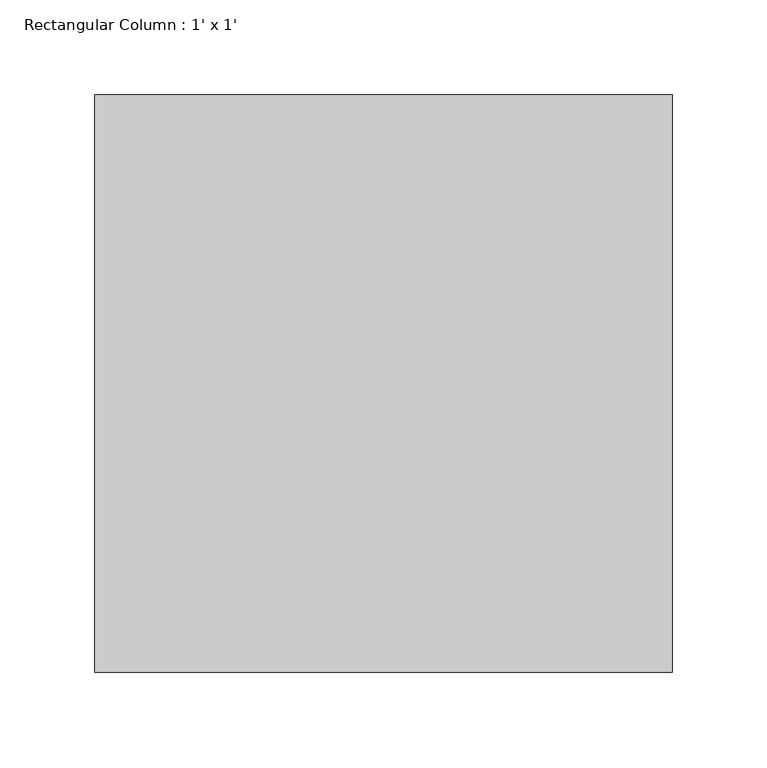
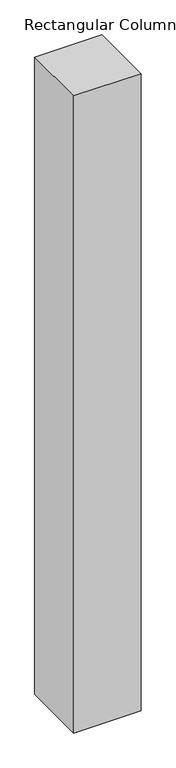
"""IFC4 building model written with IfcOpenShell, lengths in millimetres: column geometry, Rectangular Column : 1' x 1'."""

from ifc_helpers import new_model, si_unit, frame, origin, place, context, project, spatial, polyline, outline, extrude, source, transform, mapped, element, save


def rectangular_column_1_x_1_0efb18cf(model_context):
    return source(origin(), model_context, "Body", "SweptSolid", [
        extrude(outline(polyline([(152.4, 152.4), (152.4, -152.4), (-152.4, -152.4), (-152.4, 152.4), (152.4, 152.4)])), frame((0.0, 0.0, 609.6), z_axis=(0.0, 0.0, 1.0), x_axis=(1.0, 0.0, 0.0)), (0.0, 0.0, 1.0), 3048.0),
    ])


if __name__ == "__main__":
    model = new_model("IFC4")
    model_context = context("Model", 3, world=origin())
    ifc_project = project(units=[si_unit("LENGTHUNIT", "METRE", prefix="MILLI")], contexts=[model_context])
    site = spatial("IfcSite", under=ifc_project)
    building = spatial("IfcBuilding", under=site)
    placement = place(None, origin())
    rectangular_column_1_x_1_shape = rectangular_column_1_x_1_0efb18cf(model_context)
    element("IfcColumn", 1, ObjectType="Rectangular Column : 1' x 1'", at=placement, inside=building, context=model_context, shape_type="MappedRepresentation", body=[
        mapped(rectangular_column_1_x_1_shape, transform((0.0, 0.0, 0.0), x_axis=(1.0, 0.0, 0.0), y_axis=(0.0, 1.0, 0.0), z_axis=(0.0, 0.0, 1.0))),
    ])
    save(model, "model.ifc")

# Revit data of these elements
# Type "Rectangular Column : 1' x 1'"
#   Assembly Code = "B1010200"
#   Depth = 1' - 0"
#   Offset Base = 0' - 0"
#   Offset Top = 0' - 0"
#   Width = 1' - 0"
#   Material = SOFT COOL PAINT
# Element 1 (IfcColumn, "Rectangular Column : 1' x 1'")
#   Materials on its faces: "SOFT COOL PAINT"
# Materials
#   "SOFT COOL PAINT": class "Generic", colour RGB 120 120 120, transparency 0, Cost = 0
